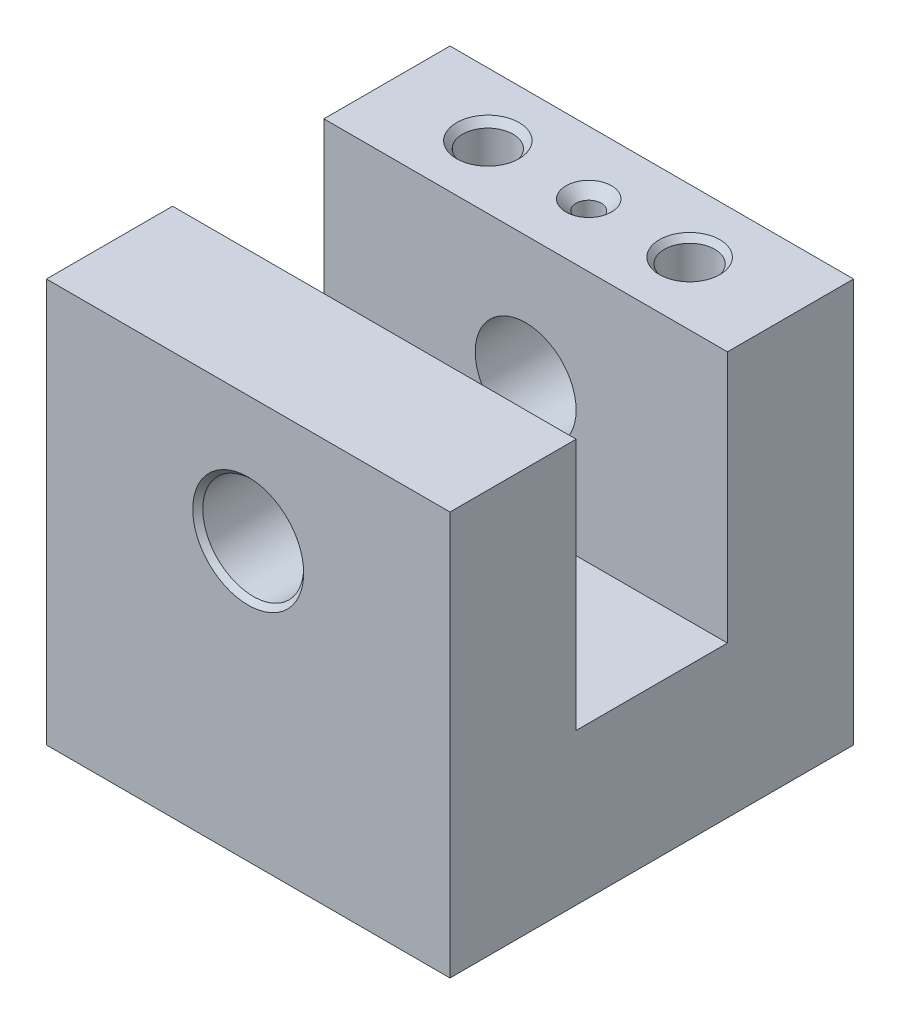
ISO-10303-21;
HEADER;
FILE_DESCRIPTION(('STEP AP214'),'2;1');
FILE_NAME('part.step','',(''),(''),'','','');
FILE_SCHEMA(('AUTOMOTIVE_DESIGN { 1 0 10303 214 1 1 1 1 }'));
ENDSEC;
DATA;
#1=APPLICATION_CONTEXT('core data for automotive mechanical design processes');
#2=APPLICATION_PROTOCOL_DEFINITION('international standard','automotive_design',2000,#1);
#3=PRODUCT_CONTEXT('',#1,'mechanical');
#4=PRODUCT('Part','Part','',(#3));
#5=PRODUCT_RELATED_PRODUCT_CATEGORY('part','',(#4));
#6=PRODUCT_DEFINITION_FORMATION('','',#4);
#7=PRODUCT_DEFINITION_CONTEXT('part definition',#1,'design');
#8=PRODUCT_DEFINITION('design','',#6,#7);
#9=PRODUCT_DEFINITION_SHAPE('','',#8);
#10=(LENGTH_UNIT() NAMED_UNIT(*) SI_UNIT(.MILLI.,.METRE.));
#11=(NAMED_UNIT(*) PLANE_ANGLE_UNIT() SI_UNIT($,.RADIAN.));
#12=(NAMED_UNIT(*) SI_UNIT($,.STERADIAN.) SOLID_ANGLE_UNIT());
#13=UNCERTAINTY_MEASURE_WITH_UNIT(LENGTH_MEASURE(1.E-05),#10,'distance_accuracy_value','');
#14=(GEOMETRIC_REPRESENTATION_CONTEXT(3) GLOBAL_UNCERTAINTY_ASSIGNED_CONTEXT((#13)) GLOBAL_UNIT_ASSIGNED_CONTEXT((#10,
#11,#12)) REPRESENTATION_CONTEXT('',''));
#15=CARTESIAN_POINT('',(0.,0.,0.));
#16=DIRECTION('',(0.,0.,1.));
#17=DIRECTION('',(1.,0.,0.));
#18=AXIS2_PLACEMENT_3D('',#15,#16,#17);
#19=CARTESIAN_POINT('',(25.4,0.,25.4));
#20=DIRECTION('',(0.,0.,-1.));
#21=DIRECTION('',(0.,1.,0.));
#22=AXIS2_PLACEMENT_3D('',#19,#20,#21);
#23=PLANE('',#22);
#24=CARTESIAN_POINT('',(0.,15.875,25.4));
#25=DIRECTION('',(0.,0.,-1.));
#26=DIRECTION('',(0.,1.,0.));
#27=AXIS2_PLACEMENT_3D('',#24,#25,#26);
#28=CIRCLE('',#27,6.98500000000002);
#29=CARTESIAN_POINT('',(0.,22.86,25.4));
#30=VERTEX_POINT('',#29);
#31=EDGE_CURVE('E11',#30,#30,#28,.T.);
#32=ORIENTED_EDGE('',*,*,#31,.T.);
#33=EDGE_LOOP('',(#32));
#34=FACE_BOUND('',#33,.T.);
#35=DIRECTION('',(0.,-1.,0.));
#36=VECTOR('',#35,1.);
#37=CARTESIAN_POINT('',(-25.4,0.,25.4));
#38=LINE('',#37,#36);
#39=CARTESIAN_POINT('',(-25.4,31.75,25.4));
#40=VERTEX_POINT('',#39);
#41=CARTESIAN_POINT('',(-25.4,-19.05,25.4));
#42=VERTEX_POINT('',#41);
#43=EDGE_CURVE('E105',#40,#42,#38,.T.);
#44=ORIENTED_EDGE('',*,*,#43,.T.);
#45=DIRECTION('',(-1.,0.,0.));
#46=VECTOR('',#45,1.);
#47=CARTESIAN_POINT('',(25.4,-19.05,25.4));
#48=LINE('',#47,#46);
#49=CARTESIAN_POINT('',(25.4,-19.05,25.4));
#50=VERTEX_POINT('',#49);
#51=EDGE_CURVE('E176',#50,#42,#48,.T.);
#52=ORIENTED_EDGE('',*,*,#51,.F.);
#53=DIRECTION('',(0.,-1.,0.));
#54=VECTOR('',#53,1.);
#55=CARTESIAN_POINT('',(25.4,0.,25.4));
#56=LINE('',#55,#54);
#57=CARTESIAN_POINT('',(25.4,31.75,25.4));
#58=VERTEX_POINT('',#57);
#59=EDGE_CURVE('E108',#58,#50,#56,.T.);
#60=ORIENTED_EDGE('',*,*,#59,.F.);
#61=DIRECTION('',(-1.,0.,0.));
#62=VECTOR('',#61,1.);
#63=CARTESIAN_POINT('',(25.4,31.75,25.4));
#64=LINE('',#63,#62);
#65=EDGE_CURVE('E144',#58,#40,#64,.T.);
#66=ORIENTED_EDGE('',*,*,#65,.T.);
#67=EDGE_LOOP('',(#44,#52,#60,#66));
#68=FACE_BOUND('',#67,.T.);
#69=ADVANCED_FACE('F50',(#34,#68),#23,.F.);
#70=CARTESIAN_POINT('',(25.4,-19.05,25.4));
#71=DIRECTION('',(0.,1.,0.));
#72=DIRECTION('',(0.,0.,1.));
#73=AXIS2_PLACEMENT_3D('',#70,#71,#72);
#74=PLANE('',#73);
#75=DIRECTION('',(0.,0.,-1.));
#76=VECTOR('',#75,1.);
#77=CARTESIAN_POINT('',(-25.4,-19.05,25.4));
#78=LINE('',#77,#76);
#79=CARTESIAN_POINT('',(-25.4,-19.05,-25.4));
#80=VERTEX_POINT('',#79);
#81=EDGE_CURVE('E148',#42,#80,#78,.T.);
#82=ORIENTED_EDGE('',*,*,#81,.T.);
#83=DIRECTION('',(-1.,0.,0.));
#84=VECTOR('',#83,1.);
#85=CARTESIAN_POINT('',(25.4,-19.05,-25.4));
#86=LINE('',#85,#84);
#87=CARTESIAN_POINT('',(25.4,-19.05,-25.4));
#88=VERTEX_POINT('',#87);
#89=EDGE_CURVE('E173',#88,#80,#86,.T.);
#90=ORIENTED_EDGE('',*,*,#89,.F.);
#91=DIRECTION('',(0.,0.,-1.));
#92=VECTOR('',#91,1.);
#93=CARTESIAN_POINT('',(25.4,-19.05,25.4));
#94=LINE('',#93,#92);
#95=EDGE_CURVE('E265',#50,#88,#94,.T.);
#96=ORIENTED_EDGE('',*,*,#95,.F.);
#97=ORIENTED_EDGE('',*,*,#51,.T.);
#98=EDGE_LOOP('',(#82,#90,#96,#97));
#99=FACE_BOUND('',#98,.T.);
#100=ADVANCED_FACE('F208',(#99),#74,.F.);
#101=CARTESIAN_POINT('',(25.4,0.,-25.4));
#102=DIRECTION('',(0.,0.,1.));
#103=DIRECTION('',(0.,-1.,0.));
#104=AXIS2_PLACEMENT_3D('',#101,#102,#103);
#105=PLANE('',#104);
#106=CARTESIAN_POINT('',(0.,15.875,-25.4));
#107=DIRECTION('',(0.,0.,1.));
#108=DIRECTION('',(0.,-1.,0.));
#109=AXIS2_PLACEMENT_3D('',#106,#107,#108);
#110=CIRCLE('',#109,6.98499999999995);
#111=CARTESIAN_POINT('',(0.,8.89000000000006,-25.4));
#112=VERTEX_POINT('',#111);
#113=EDGE_CURVE('E184',#112,#112,#110,.T.);
#114=ORIENTED_EDGE('',*,*,#113,.T.);
#115=EDGE_LOOP('',(#114));
#116=FACE_BOUND('',#115,.T.);
#117=DIRECTION('',(0.,1.,0.));
#118=VECTOR('',#117,1.);
#119=CARTESIAN_POINT('',(-25.4,0.,-25.4));
#120=LINE('',#119,#118);
#121=CARTESIAN_POINT('',(-25.4,31.75,-25.4));
#122=VERTEX_POINT('',#121);
#123=EDGE_CURVE('E153',#80,#122,#120,.T.);
#124=ORIENTED_EDGE('',*,*,#123,.T.);
#125=DIRECTION('',(-1.,0.,0.));
#126=VECTOR('',#125,1.);
#127=CARTESIAN_POINT('',(25.4,31.75,-25.4));
#128=LINE('',#127,#126);
#129=CARTESIAN_POINT('',(25.4,31.75,-25.4));
#130=VERTEX_POINT('',#129);
#131=EDGE_CURVE('E167',#130,#122,#128,.T.);
#132=ORIENTED_EDGE('',*,*,#131,.F.);
#133=DIRECTION('',(0.,1.,0.));
#134=VECTOR('',#133,1.);
#135=CARTESIAN_POINT('',(25.4,0.,-25.4));
#136=LINE('',#135,#134);
#137=EDGE_CURVE('E264',#88,#130,#136,.T.);
#138=ORIENTED_EDGE('',*,*,#137,.F.);
#139=ORIENTED_EDGE('',*,*,#89,.T.);
#140=EDGE_LOOP('',(#124,#132,#138,#139));
#141=FACE_BOUND('',#140,.T.);
#142=ADVANCED_FACE('F218',(#116,#141),#105,.F.);
#143=CARTESIAN_POINT('',(25.4,31.75,-25.4));
#144=DIRECTION('',(0.,-1.,0.));
#145=DIRECTION('',(0.,0.,-1.));
#146=AXIS2_PLACEMENT_3D('',#143,#144,#145);
#147=PLANE('',#146);
#148=CARTESIAN_POINT('',(-12.7,31.75,-17.4625));
#149=DIRECTION('',(0.,1.,0.));
#150=DIRECTION('',(0.,0.,1.));
#151=AXIS2_PLACEMENT_3D('',#148,#149,#150);
#152=CIRCLE('',#151,3.937);
#153=CARTESIAN_POINT('',(-12.7,31.75,-13.5255));
#154=VERTEX_POINT('',#153);
#155=EDGE_CURVE('E346',#154,#154,#152,.T.);
#156=ORIENTED_EDGE('',*,*,#155,.F.);
#157=EDGE_LOOP('',(#156));
#158=FACE_BOUND('',#157,.T.);
#159=CARTESIAN_POINT('',(12.7,31.75,-17.4625));
#160=DIRECTION('',(0.,1.,0.));
#161=DIRECTION('',(0.,0.,1.));
#162=AXIS2_PLACEMENT_3D('',#159,#160,#161);
#163=CIRCLE('',#162,3.81);
#164=CARTESIAN_POINT('',(12.7,31.75,-13.6525));
#165=VERTEX_POINT('',#164);
#166=EDGE_CURVE('E370',#165,#165,#163,.T.);
#167=ORIENTED_EDGE('',*,*,#166,.F.);
#168=EDGE_LOOP('',(#167));
#169=FACE_BOUND('',#168,.T.);
#170=CARTESIAN_POINT('',(0.,31.75,-17.4625));
#171=DIRECTION('',(0.,-1.,0.));
#172=DIRECTION('',(0.,0.,-1.));
#173=AXIS2_PLACEMENT_3D('',#170,#171,#172);
#174=CIRCLE('',#173,2.87019999999999);
#175=CARTESIAN_POINT('',(0.,31.75,-20.3327));
#176=VERTEX_POINT('',#175);
#177=EDGE_CURVE('E185',#176,#176,#174,.T.);
#178=ORIENTED_EDGE('',*,*,#177,.T.);
#179=EDGE_LOOP('',(#178));
#180=FACE_BOUND('',#179,.T.);
#181=DIRECTION('',(0.,0.,1.));
#182=VECTOR('',#181,1.);
#183=CARTESIAN_POINT('',(-25.4,31.75,-25.4));
#184=LINE('',#183,#182);
#185=CARTESIAN_POINT('',(-25.4,31.75,-9.525));
#186=VERTEX_POINT('',#185);
#187=EDGE_CURVE('E151',#122,#186,#184,.T.);
#188=ORIENTED_EDGE('',*,*,#187,.T.);
#189=DIRECTION('',(-1.,0.,0.));
#190=VECTOR('',#189,1.);
#191=CARTESIAN_POINT('',(25.4,31.75,-9.525));
#192=LINE('',#191,#190);
#193=CARTESIAN_POINT('',(25.4,31.75,-9.525));
#194=VERTEX_POINT('',#193);
#195=EDGE_CURVE('E170',#194,#186,#192,.T.);
#196=ORIENTED_EDGE('',*,*,#195,.F.);
#197=DIRECTION('',(0.,0.,1.));
#198=VECTOR('',#197,1.);
#199=CARTESIAN_POINT('',(25.4,31.75,-25.4));
#200=LINE('',#199,#198);
#201=EDGE_CURVE('E266',#130,#194,#200,.T.);
#202=ORIENTED_EDGE('',*,*,#201,.F.);
#203=ORIENTED_EDGE('',*,*,#131,.T.);
#204=EDGE_LOOP('',(#188,#196,#202,#203));
#205=FACE_BOUND('',#204,.T.);
#206=ADVANCED_FACE('F275',(#158,#169,#180,#205),#147,.F.);
#207=CARTESIAN_POINT('',(25.4,0.,-9.525));
#208=DIRECTION('',(0.,0.,-1.));
#209=DIRECTION('',(-1.,0.,0.));
#210=AXIS2_PLACEMENT_3D('',#207,#208,#209);
#211=PLANE('',#210);
#212=CARTESIAN_POINT('',(0.,15.875,-9.52500000000001));
#213=DIRECTION('',(0.,0.,-1.));
#214=DIRECTION('',(-1.,0.,0.));
#215=AXIS2_PLACEMENT_3D('',#212,#213,#214);
#216=CIRCLE('',#215,6.34999999999999);
#217=CARTESIAN_POINT('',(-6.34999999999999,15.875,-9.52500000000001));
#218=VERTEX_POINT('',#217);
#219=EDGE_CURVE('E186',#218,#218,#216,.T.);
#220=ORIENTED_EDGE('',*,*,#219,.T.);
#221=EDGE_LOOP('',(#220));
#222=FACE_BOUND('',#221,.T.);
#223=DIRECTION('',(0.,-1.,0.));
#224=VECTOR('',#223,1.);
#225=CARTESIAN_POINT('',(-25.4,0.,-9.525));
#226=LINE('',#225,#224);
#227=CARTESIAN_POINT('',(-25.4,0.,-9.525));
#228=VERTEX_POINT('',#227);
#229=EDGE_CURVE('E160',#186,#228,#226,.T.);
#230=ORIENTED_EDGE('',*,*,#229,.T.);
#231=DIRECTION('',(-1.,0.,0.));
#232=VECTOR('',#231,1.);
#233=CARTESIAN_POINT('',(25.4,0.,-9.525));
#234=LINE('',#233,#232);
#235=CARTESIAN_POINT('',(25.4,0.,-9.525));
#236=VERTEX_POINT('',#235);
#237=EDGE_CURVE('E137',#236,#228,#234,.T.);
#238=ORIENTED_EDGE('',*,*,#237,.F.);
#239=DIRECTION('',(0.,-1.,0.));
#240=VECTOR('',#239,1.);
#241=CARTESIAN_POINT('',(25.4,0.,-9.525));
#242=LINE('',#241,#240);
#243=EDGE_CURVE('E127',#194,#236,#242,.T.);
#244=ORIENTED_EDGE('',*,*,#243,.F.);
#245=ORIENTED_EDGE('',*,*,#195,.T.);
#246=EDGE_LOOP('',(#230,#238,#244,#245));
#247=FACE_BOUND('',#246,.T.);
#248=ADVANCED_FACE('F279',(#222,#247),#211,.F.);
#249=CARTESIAN_POINT('',(25.4,0.,9.525));
#250=DIRECTION('',(0.,-1.,0.));
#251=DIRECTION('',(0.,0.,-1.));
#252=AXIS2_PLACEMENT_3D('',#249,#250,#251);
#253=PLANE('',#252);
#254=DIRECTION('',(0.,0.,1.));
#255=VECTOR('',#254,1.);
#256=CARTESIAN_POINT('',(-25.4,0.,9.525));
#257=LINE('',#256,#255);
#258=CARTESIAN_POINT('',(-25.4,0.,9.525));
#259=VERTEX_POINT('',#258);
#260=EDGE_CURVE('E138',#228,#259,#257,.T.);
#261=ORIENTED_EDGE('',*,*,#260,.T.);
#262=DIRECTION('',(-1.,0.,0.));
#263=VECTOR('',#262,1.);
#264=CARTESIAN_POINT('',(25.4,0.,9.525));
#265=LINE('',#264,#263);
#266=CARTESIAN_POINT('',(25.4,0.,9.525));
#267=VERTEX_POINT('',#266);
#268=EDGE_CURVE('E131',#267,#259,#265,.T.);
#269=ORIENTED_EDGE('',*,*,#268,.F.);
#270=DIRECTION('',(0.,0.,1.));
#271=VECTOR('',#270,1.);
#272=CARTESIAN_POINT('',(25.4,0.,9.525));
#273=LINE('',#272,#271);
#274=EDGE_CURVE('E121',#236,#267,#273,.T.);
#275=ORIENTED_EDGE('',*,*,#274,.F.);
#276=ORIENTED_EDGE('',*,*,#237,.T.);
#277=EDGE_LOOP('',(#261,#269,#275,#276));
#278=FACE_BOUND('',#277,.T.);
#279=ADVANCED_FACE('F136',(#278),#253,.F.);
#280=CARTESIAN_POINT('',(25.4,0.,9.525));
#281=DIRECTION('',(0.,0.,1.));
#282=DIRECTION('',(1.,0.,0.));
#283=AXIS2_PLACEMENT_3D('',#280,#281,#282);
#284=PLANE('',#283);
#285=CARTESIAN_POINT('',(0.,15.875,9.525));
#286=DIRECTION('',(0.,0.,1.));
#287=DIRECTION('',(1.,0.,0.));
#288=AXIS2_PLACEMENT_3D('',#285,#286,#287);
#289=CIRCLE('',#288,6.34999999999999);
#290=CARTESIAN_POINT('',(6.34999999999999,15.875,9.525));
#291=VERTEX_POINT('',#290);
#292=EDGE_CURVE('E187',#291,#291,#289,.T.);
#293=ORIENTED_EDGE('',*,*,#292,.T.);
#294=EDGE_LOOP('',(#293));
#295=FACE_BOUND('',#294,.T.);
#296=DIRECTION('',(0.,1.,0.));
#297=VECTOR('',#296,1.);
#298=CARTESIAN_POINT('',(-25.4,0.,9.525));
#299=LINE('',#298,#297);
#300=CARTESIAN_POINT('',(-25.4,31.75,9.525));
#301=VERTEX_POINT('',#300);
#302=EDGE_CURVE('E94',#259,#301,#299,.T.);
#303=ORIENTED_EDGE('',*,*,#302,.T.);
#304=DIRECTION('',(-1.,0.,0.));
#305=VECTOR('',#304,1.);
#306=CARTESIAN_POINT('',(25.4,31.75,9.525));
#307=LINE('',#306,#305);
#308=CARTESIAN_POINT('',(25.4,31.75,9.525));
#309=VERTEX_POINT('',#308);
#310=EDGE_CURVE('E139',#309,#301,#307,.T.);
#311=ORIENTED_EDGE('',*,*,#310,.F.);
#312=DIRECTION('',(0.,1.,0.));
#313=VECTOR('',#312,1.);
#314=CARTESIAN_POINT('',(25.4,0.,9.525));
#315=LINE('',#314,#313);
#316=EDGE_CURVE('E130',#267,#309,#315,.T.);
#317=ORIENTED_EDGE('',*,*,#316,.F.);
#318=ORIENTED_EDGE('',*,*,#268,.T.);
#319=EDGE_LOOP('',(#303,#311,#317,#318));
#320=FACE_BOUND('',#319,.T.);
#321=ADVANCED_FACE('F145',(#295,#320),#284,.F.);
#322=CARTESIAN_POINT('',(25.4,31.75,25.4));
#323=DIRECTION('',(0.,-1.,0.));
#324=DIRECTION('',(0.,0.,-1.));
#325=AXIS2_PLACEMENT_3D('',#322,#323,#324);
#326=PLANE('',#325);
#327=DIRECTION('',(0.,0.,1.));
#328=VECTOR('',#327,1.);
#329=CARTESIAN_POINT('',(-25.4,31.75,25.4));
#330=LINE('',#329,#328);
#331=EDGE_CURVE('E163',#301,#40,#330,.T.);
#332=ORIENTED_EDGE('',*,*,#331,.T.);
#333=ORIENTED_EDGE('',*,*,#65,.F.);
#334=DIRECTION('',(0.,0.,1.));
#335=VECTOR('',#334,1.);
#336=CARTESIAN_POINT('',(25.4,31.75,25.4));
#337=LINE('',#336,#335);
#338=EDGE_CURVE('E62',#309,#58,#337,.T.);
#339=ORIENTED_EDGE('',*,*,#338,.F.);
#340=ORIENTED_EDGE('',*,*,#310,.T.);
#341=EDGE_LOOP('',(#332,#333,#339,#340));
#342=FACE_BOUND('',#341,.T.);
#343=ADVANCED_FACE('F278',(#342),#326,.F.);
#344=CARTESIAN_POINT('',(25.4,0.,0.));
#345=DIRECTION('',(-1.,0.,0.));
#346=DIRECTION('',(0.,0.,1.));
#347=AXIS2_PLACEMENT_3D('',#344,#345,#346);
#348=PLANE('',#347);
#349=ORIENTED_EDGE('',*,*,#59,.T.);
#350=ORIENTED_EDGE('',*,*,#95,.T.);
#351=ORIENTED_EDGE('',*,*,#137,.T.);
#352=ORIENTED_EDGE('',*,*,#201,.T.);
#353=ORIENTED_EDGE('',*,*,#243,.T.);
#354=ORIENTED_EDGE('',*,*,#274,.T.);
#355=ORIENTED_EDGE('',*,*,#316,.T.);
#356=ORIENTED_EDGE('',*,*,#338,.T.);
#357=EDGE_LOOP('',(#349,#350,#351,#352,#353,#354,#355,#356));
#358=FACE_BOUND('',#357,.T.);
#359=ADVANCED_FACE('F129',(#358),#348,.F.);
#360=CARTESIAN_POINT('',(-25.4,0.,0.));
#361=DIRECTION('',(-1.,0.,0.));
#362=DIRECTION('',(0.,0.,1.));
#363=AXIS2_PLACEMENT_3D('',#360,#361,#362);
#364=PLANE('',#363);
#365=ORIENTED_EDGE('',*,*,#43,.F.);
#366=ORIENTED_EDGE('',*,*,#331,.F.);
#367=ORIENTED_EDGE('',*,*,#302,.F.);
#368=ORIENTED_EDGE('',*,*,#260,.F.);
#369=ORIENTED_EDGE('',*,*,#229,.F.);
#370=ORIENTED_EDGE('',*,*,#187,.F.);
#371=ORIENTED_EDGE('',*,*,#123,.F.);
#372=ORIENTED_EDGE('',*,*,#81,.F.);
#373=EDGE_LOOP('',(#365,#366,#367,#368,#369,#370,#371,#372));
#374=FACE_BOUND('',#373,.T.);
#375=ADVANCED_FACE('F276',(#374),#364,.T.);
#376=CARTESIAN_POINT('',(0.,24.13,-17.4625));
#377=DIRECTION('',(0.,1.,0.));
#378=DIRECTION('',(0.,0.,1.));
#379=AXIS2_PLACEMENT_3D('',#376,#377,#378);
#380=CONICAL_SURFACE('',#379,1.6002,1.02974425867665);
#381=CARTESIAN_POINT('',(0.,23.1685028374321,-17.4625));
#382=VERTEX_POINT('',#381);
#383=VERTEX_LOOP('',#382);
#384=FACE_BOUND('',#383,.T.);
#385=CARTESIAN_POINT('',(0.,24.13,-17.4625));
#386=DIRECTION('',(0.,1.,0.));
#387=DIRECTION('',(0.,0.,1.));
#388=AXIS2_PLACEMENT_3D('',#385,#386,#387);
#389=CIRCLE('',#388,1.6002);
#390=CARTESIAN_POINT('',(0.,24.13,-15.8623));
#391=VERTEX_POINT('',#390);
#392=EDGE_CURVE('E147',#391,#391,#389,.T.);
#393=ORIENTED_EDGE('',*,*,#392,.T.);
#394=EDGE_LOOP('',(#393));
#395=FACE_BOUND('',#394,.T.);
#396=ADVANCED_FACE('F242',(#384,#395),#380,.F.);
#397=CARTESIAN_POINT('',(0.,31.75,-17.4625));
#398=DIRECTION('',(0.,1.,0.));
#399=DIRECTION('',(0.,0.,1.));
#400=AXIS2_PLACEMENT_3D('',#397,#398,#399);
#401=CYLINDRICAL_SURFACE('',#400,1.6002);
#402=CARTESIAN_POINT('',(0.,30.48,-17.4625));
#403=DIRECTION('',(0.,-1.,0.));
#404=DIRECTION('',(0.,0.,-1.));
#405=AXIS2_PLACEMENT_3D('',#402,#403,#404);
#406=CIRCLE('',#405,1.6002);
#407=CARTESIAN_POINT('',(0.,30.48,-19.0627));
#408=VERTEX_POINT('',#407);
#409=EDGE_CURVE('E177',#408,#408,#406,.F.);
#410=ORIENTED_EDGE('',*,*,#409,.T.);
#411=EDGE_LOOP('',(#410));
#412=FACE_BOUND('',#411,.T.);
#413=ORIENTED_EDGE('',*,*,#392,.F.);
#414=EDGE_LOOP('',(#413));
#415=FACE_BOUND('',#414,.T.);
#416=ADVANCED_FACE('F233',(#412,#415),#401,.F.);
#417=CARTESIAN_POINT('',(0.,30.48,-17.4625));
#418=DIRECTION('',(0.,1.,0.));
#419=DIRECTION('',(0.,0.,1.));
#420=AXIS2_PLACEMENT_3D('',#417,#418,#419);
#421=CONICAL_SURFACE('',#420,1.6002,0.785398163397451);
#422=ORIENTED_EDGE('',*,*,#177,.F.);
#423=EDGE_LOOP('',(#422));
#424=FACE_BOUND('',#423,.T.);
#425=ORIENTED_EDGE('',*,*,#409,.F.);
#426=EDGE_LOOP('',(#425));
#427=FACE_BOUND('',#426,.T.);
#428=ADVANCED_FACE('F224',(#424,#427),#421,.F.);
#429=CARTESIAN_POINT('',(12.7,15.24,-17.4625));
#430=DIRECTION('',(0.,1.,0.));
#431=DIRECTION('',(0.,0.,1.));
#432=AXIS2_PLACEMENT_3D('',#429,#430,#431);
#433=CONICAL_SURFACE('',#432,2.55269999999999,0.785398163397445);
#434=CARTESIAN_POINT('',(12.7,12.6873,-17.4625));
#435=VERTEX_POINT('',#434);
#436=VERTEX_LOOP('',#435);
#437=FACE_BOUND('',#436,.T.);
#438=CARTESIAN_POINT('',(12.7,15.24,-17.4625));
#439=DIRECTION('',(0.,1.,0.));
#440=DIRECTION('',(0.,0.,1.));
#441=AXIS2_PLACEMENT_3D('',#438,#439,#440);
#442=CIRCLE('',#441,2.55269999999999);
#443=CARTESIAN_POINT('',(12.7,15.24,-14.9098));
#444=VERTEX_POINT('',#443);
#445=EDGE_CURVE('E251',#444,#444,#442,.T.);
#446=ORIENTED_EDGE('',*,*,#445,.T.);
#447=EDGE_LOOP('',(#446));
#448=FACE_BOUND('',#447,.T.);
#449=ADVANCED_FACE('F229',(#437,#448),#433,.F.);
#450=CARTESIAN_POINT('',(12.7,31.75,-17.4625));
#451=DIRECTION('',(0.,1.,0.));
#452=DIRECTION('',(0.,0.,1.));
#453=AXIS2_PLACEMENT_3D('',#450,#451,#452);
#454=CYLINDRICAL_SURFACE('',#453,2.55269999999999);
#455=ORIENTED_EDGE('',*,*,#445,.F.);
#456=EDGE_LOOP('',(#455));
#457=FACE_BOUND('',#456,.T.);
#458=CARTESIAN_POINT('',(12.7,19.05,-17.4625));
#459=DIRECTION('',(0.,1.,0.));
#460=DIRECTION('',(0.,0.,1.));
#461=AXIS2_PLACEMENT_3D('',#458,#459,#460);
#462=CIRCLE('',#461,2.55269999999999);
#463=CARTESIAN_POINT('',(12.7,19.05,-14.9098));
#464=VERTEX_POINT('',#463);
#465=EDGE_CURVE('E256',#464,#464,#462,.T.);
#466=ORIENTED_EDGE('',*,*,#465,.T.);
#467=EDGE_LOOP('',(#466));
#468=FACE_BOUND('',#467,.T.);
#469=ADVANCED_FACE('F241',(#457,#468),#454,.F.);
#470=CARTESIAN_POINT('',(15.2527,19.05,-17.4625));
#471=DIRECTION('',(0.,-1.,0.));
#472=DIRECTION('',(0.,0.,-1.));
#473=AXIS2_PLACEMENT_3D('',#470,#471,#472);
#474=PLANE('',#473);
#475=ORIENTED_EDGE('',*,*,#465,.F.);
#476=EDGE_LOOP('',(#475));
#477=FACE_BOUND('',#476,.T.);
#478=CARTESIAN_POINT('',(12.7,19.05,-17.4625));
#479=DIRECTION('',(0.,1.,0.));
#480=DIRECTION('',(0.,0.,1.));
#481=AXIS2_PLACEMENT_3D('',#478,#479,#480);
#482=CIRCLE('',#481,3.17499999999999);
#483=CARTESIAN_POINT('',(12.7,19.05,-14.2875));
#484=VERTEX_POINT('',#483);
#485=EDGE_CURVE('E373',#484,#484,#482,.T.);
#486=ORIENTED_EDGE('',*,*,#485,.T.);
#487=EDGE_LOOP('',(#486));
#488=FACE_BOUND('',#487,.T.);
#489=ADVANCED_FACE('F307',(#477,#488),#474,.F.);
#490=CARTESIAN_POINT('',(12.7,31.75,-17.4625));
#491=DIRECTION('',(0.,1.,0.));
#492=DIRECTION('',(0.,0.,1.));
#493=AXIS2_PLACEMENT_3D('',#490,#491,#492);
#494=CYLINDRICAL_SURFACE('',#493,3.175);
#495=ORIENTED_EDGE('',*,*,#485,.F.);
#496=EDGE_LOOP('',(#495));
#497=FACE_BOUND('',#496,.T.);
#498=CARTESIAN_POINT('',(12.7,31.0195160614147,-17.4625));
#499=DIRECTION('',(0.,1.,0.));
#500=DIRECTION('',(0.,0.,1.));
#501=AXIS2_PLACEMENT_3D('',#498,#499,#500);
#502=CIRCLE('',#501,3.175);
#503=CARTESIAN_POINT('',(12.7,31.0195160614147,-14.2875));
#504=VERTEX_POINT('',#503);
#505=EDGE_CURVE('E369',#504,#504,#502,.T.);
#506=ORIENTED_EDGE('',*,*,#505,.T.);
#507=EDGE_LOOP('',(#506));
#508=FACE_BOUND('',#507,.T.);
#509=ADVANCED_FACE('F312',(#497,#508),#494,.F.);
#510=CARTESIAN_POINT('',(12.7,31.75,-17.4625));
#511=DIRECTION('',(0.,1.,0.));
#512=DIRECTION('',(0.,0.,1.));
#513=AXIS2_PLACEMENT_3D('',#510,#511,#512);
#514=CONICAL_SURFACE('',#513,3.81,0.715584993317677);
#515=ORIENTED_EDGE('',*,*,#505,.F.);
#516=EDGE_LOOP('',(#515));
#517=FACE_BOUND('',#516,.T.);
#518=ORIENTED_EDGE('',*,*,#166,.T.);
#519=EDGE_LOOP('',(#518));
#520=FACE_BOUND('',#519,.T.);
#521=ADVANCED_FACE('F320',(#517,#520),#514,.F.);
#522=CARTESIAN_POINT('',(-12.7,15.24,-17.4625));
#523=DIRECTION('',(0.,1.,0.));
#524=DIRECTION('',(0.,0.,1.));
#525=AXIS2_PLACEMENT_3D('',#522,#523,#524);
#526=CONICAL_SURFACE('',#525,2.55269999999999,0.785398163397446);
#527=CARTESIAN_POINT('',(-12.7,12.6873,-17.4625));
#528=VERTEX_POINT('',#527);
#529=VERTEX_LOOP('',#528);
#530=FACE_BOUND('',#529,.T.);
#531=CARTESIAN_POINT('',(-12.7,15.24,-17.4625));
#532=DIRECTION('',(0.,1.,0.));
#533=DIRECTION('',(0.,0.,1.));
#534=AXIS2_PLACEMENT_3D('',#531,#532,#533);
#535=CIRCLE('',#534,2.55269999999999);
#536=CARTESIAN_POINT('',(-12.7,15.24,-14.9098));
#537=VERTEX_POINT('',#536);
#538=EDGE_CURVE('E364',#537,#537,#535,.T.);
#539=ORIENTED_EDGE('',*,*,#538,.T.);
#540=EDGE_LOOP('',(#539));
#541=FACE_BOUND('',#540,.T.);
#542=ADVANCED_FACE('F324',(#530,#541),#526,.F.);
#543=CARTESIAN_POINT('',(-12.7,31.75,-17.4625));
#544=DIRECTION('',(0.,1.,0.));
#545=DIRECTION('',(0.,0.,1.));
#546=AXIS2_PLACEMENT_3D('',#543,#544,#545);
#547=CYLINDRICAL_SURFACE('',#546,2.55269999999999);
#548=ORIENTED_EDGE('',*,*,#538,.F.);
#549=EDGE_LOOP('',(#548));
#550=FACE_BOUND('',#549,.T.);
#551=CARTESIAN_POINT('',(-12.7,19.05,-17.4625));
#552=DIRECTION('',(0.,1.,0.));
#553=DIRECTION('',(0.,0.,1.));
#554=AXIS2_PLACEMENT_3D('',#551,#552,#553);
#555=CIRCLE('',#554,2.55269999999999);
#556=CARTESIAN_POINT('',(-12.7,19.05,-14.9098));
#557=VERTEX_POINT('',#556);
#558=EDGE_CURVE('E363',#557,#557,#555,.T.);
#559=ORIENTED_EDGE('',*,*,#558,.T.);
#560=EDGE_LOOP('',(#559));
#561=FACE_BOUND('',#560,.T.);
#562=ADVANCED_FACE('F322',(#550,#561),#547,.F.);
#563=CARTESIAN_POINT('',(-10.1473,19.05,-17.4625));
#564=DIRECTION('',(0.,-1.,0.));
#565=DIRECTION('',(0.,0.,-1.));
#566=AXIS2_PLACEMENT_3D('',#563,#564,#565);
#567=PLANE('',#566);
#568=ORIENTED_EDGE('',*,*,#558,.F.);
#569=EDGE_LOOP('',(#568));
#570=FACE_BOUND('',#569,.T.);
#571=CARTESIAN_POINT('',(-12.7,19.05,-17.4625));
#572=DIRECTION('',(0.,1.,0.));
#573=DIRECTION('',(0.,0.,1.));
#574=AXIS2_PLACEMENT_3D('',#571,#572,#573);
#575=CIRCLE('',#574,3.17499999999999);
#576=CARTESIAN_POINT('',(-12.7,19.05,-14.2875));
#577=VERTEX_POINT('',#576);
#578=EDGE_CURVE('E356',#577,#577,#575,.T.);
#579=ORIENTED_EDGE('',*,*,#578,.T.);
#580=EDGE_LOOP('',(#579));
#581=FACE_BOUND('',#580,.T.);
#582=ADVANCED_FACE('F329',(#570,#581),#567,.F.);
#583=CARTESIAN_POINT('',(-12.7,31.75,-17.4625));
#584=DIRECTION('',(0.,1.,0.));
#585=DIRECTION('',(0.,0.,1.));
#586=AXIS2_PLACEMENT_3D('',#583,#584,#585);
#587=CYLINDRICAL_SURFACE('',#586,3.17499999999999);
#588=ORIENTED_EDGE('',*,*,#578,.F.);
#589=EDGE_LOOP('',(#588));
#590=FACE_BOUND('',#589,.T.);
#591=CARTESIAN_POINT('',(-12.7,30.8734192736976,-17.4625));
#592=DIRECTION('',(0.,1.,0.));
#593=DIRECTION('',(0.,0.,1.));
#594=AXIS2_PLACEMENT_3D('',#591,#592,#593);
#595=CIRCLE('',#594,3.175);
#596=CARTESIAN_POINT('',(-12.7,30.8734192736976,-14.2875));
#597=VERTEX_POINT('',#596);
#598=EDGE_CURVE('E353',#597,#597,#595,.T.);
#599=ORIENTED_EDGE('',*,*,#598,.T.);
#600=EDGE_LOOP('',(#599));
#601=FACE_BOUND('',#600,.T.);
#602=ADVANCED_FACE('F333',(#590,#601),#587,.F.);
#603=CARTESIAN_POINT('',(-12.7,31.75,-17.4625));
#604=DIRECTION('',(0.,1.,0.));
#605=DIRECTION('',(0.,0.,1.));
#606=AXIS2_PLACEMENT_3D('',#603,#604,#605);
#607=CONICAL_SURFACE('',#606,3.937,0.715584993317676);
#608=ORIENTED_EDGE('',*,*,#598,.F.);
#609=EDGE_LOOP('',(#608));
#610=FACE_BOUND('',#609,.T.);
#611=ORIENTED_EDGE('',*,*,#155,.T.);
#612=EDGE_LOOP('',(#611));
#613=FACE_BOUND('',#612,.T.);
#614=ADVANCED_FACE('F340',(#610,#613),#607,.F.);
#615=CARTESIAN_POINT('',(0.,15.875,25.4));
#616=DIRECTION('',(0.,0.,1.));
#617=DIRECTION('',(0.,-1.,0.));
#618=AXIS2_PLACEMENT_3D('',#615,#616,#617);
#619=CYLINDRICAL_SURFACE('',#618,6.34999999999999);
#620=CARTESIAN_POINT('',(0.,15.875,24.765));
#621=DIRECTION('',(0.,0.,-1.));
#622=DIRECTION('',(-1.,0.,0.));
#623=AXIS2_PLACEMENT_3D('',#620,#621,#622);
#624=CIRCLE('',#623,6.34999999999999);
#625=CARTESIAN_POINT('',(-6.34999999999999,15.875,24.765));
#626=VERTEX_POINT('',#625);
#627=EDGE_CURVE('E60',#626,#626,#624,.F.);
#628=ORIENTED_EDGE('',*,*,#627,.T.);
#629=EDGE_LOOP('',(#628));
#630=FACE_BOUND('',#629,.T.);
#631=ORIENTED_EDGE('',*,*,#292,.F.);
#632=EDGE_LOOP('',(#631));
#633=FACE_BOUND('',#632,.T.);
#634=ADVANCED_FACE('F200',(#630,#633),#619,.F.);
#635=CARTESIAN_POINT('',(0.,15.875,-24.765));
#636=DIRECTION('',(0.,0.,1.));
#637=DIRECTION('',(1.,0.,0.));
#638=AXIS2_PLACEMENT_3D('',#635,#636,#637);
#639=CIRCLE('',#638,6.34999999999999);
#640=CARTESIAN_POINT('',(6.34999999999999,15.875,-24.765));
#641=VERTEX_POINT('',#640);
#642=EDGE_CURVE('E191',#641,#641,#639,.F.);
#643=ORIENTED_EDGE('',*,*,#642,.T.);
#644=EDGE_LOOP('',(#643));
#645=FACE_BOUND('',#644,.T.);
#646=ORIENTED_EDGE('',*,*,#219,.F.);
#647=EDGE_LOOP('',(#646));
#648=FACE_BOUND('',#647,.T.);
#649=ADVANCED_FACE('F207',(#645,#648),#619,.F.);
#650=CARTESIAN_POINT('',(0.,15.875,-25.4));
#651=DIRECTION('',(0.,0.,-1.));
#652=DIRECTION('',(-1.,0.,0.));
#653=AXIS2_PLACEMENT_3D('',#650,#651,#652);
#654=CONICAL_SURFACE('',#653,6.98499999999995,0.785398163397442);
#655=ORIENTED_EDGE('',*,*,#642,.F.);
#656=EDGE_LOOP('',(#655));
#657=FACE_BOUND('',#656,.T.);
#658=ORIENTED_EDGE('',*,*,#113,.F.);
#659=EDGE_LOOP('',(#658));
#660=FACE_BOUND('',#659,.T.);
#661=ADVANCED_FACE('F201',(#657,#660),#654,.F.);
#662=CARTESIAN_POINT('',(0.,15.875,24.765));
#663=DIRECTION('',(0.,0.,1.));
#664=DIRECTION('',(1.,0.,0.));
#665=AXIS2_PLACEMENT_3D('',#662,#663,#664);
#666=CONICAL_SURFACE('',#665,6.34999999999999,0.785398163397459);
#667=ORIENTED_EDGE('',*,*,#31,.F.);
#668=EDGE_LOOP('',(#667));
#669=FACE_BOUND('',#668,.T.);
#670=ORIENTED_EDGE('',*,*,#627,.F.);
#671=EDGE_LOOP('',(#670));
#672=FACE_BOUND('',#671,.T.);
#673=ADVANCED_FACE('F49',(#669,#672),#666,.F.);
#674=CLOSED_SHELL('',(#69,#100,#142,#206,#248,#279,#321,#343,#359,#375,#396,#416,#428,#449,#469,
#489,#509,#521,#542,#562,#582,#602,#614,#634,#649,#661,#673));
#675=MANIFOLD_SOLID_BREP('B2',#674);
#676=ADVANCED_BREP_SHAPE_REPRESENTATION('',(#18,#675),#14);
#677=SHAPE_DEFINITION_REPRESENTATION(#9,#676);
ENDSEC;
END-ISO-10303-21;
